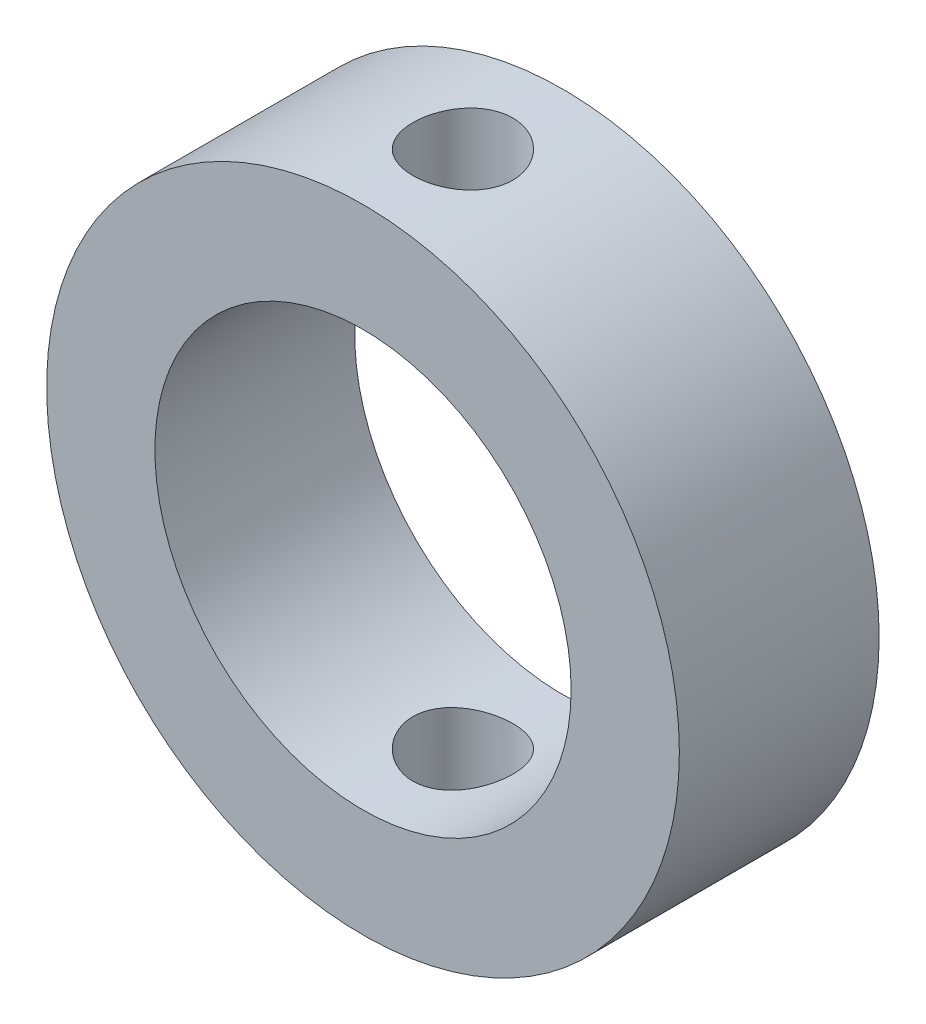
ISO-10303-21;
HEADER;
FILE_DESCRIPTION(('STEP AP214'),'2;1');
FILE_NAME('part.step','',(''),(''),'','','');
FILE_SCHEMA(('AUTOMOTIVE_DESIGN { 1 0 10303 214 1 1 1 1 }'));
ENDSEC;
DATA;
#1=APPLICATION_CONTEXT('core data for automotive mechanical design processes');
#2=APPLICATION_PROTOCOL_DEFINITION('international standard','automotive_design',2000,#1);
#3=PRODUCT_CONTEXT('',#1,'mechanical');
#4=PRODUCT('Part','Part','',(#3));
#5=PRODUCT_RELATED_PRODUCT_CATEGORY('part','',(#4));
#6=PRODUCT_DEFINITION_FORMATION('','',#4);
#7=PRODUCT_DEFINITION_CONTEXT('part definition',#1,'design');
#8=PRODUCT_DEFINITION('design','',#6,#7);
#9=PRODUCT_DEFINITION_SHAPE('','',#8);
#10=(LENGTH_UNIT() NAMED_UNIT(*) SI_UNIT(.MILLI.,.METRE.));
#11=(NAMED_UNIT(*) PLANE_ANGLE_UNIT() SI_UNIT($,.RADIAN.));
#12=(NAMED_UNIT(*) SI_UNIT($,.STERADIAN.) SOLID_ANGLE_UNIT());
#13=UNCERTAINTY_MEASURE_WITH_UNIT(LENGTH_MEASURE(1.E-05),#10,'distance_accuracy_value','');
#14=(GEOMETRIC_REPRESENTATION_CONTEXT(3) GLOBAL_UNCERTAINTY_ASSIGNED_CONTEXT((#13)) GLOBAL_UNIT_ASSIGNED_CONTEXT((#10,
#11,#12)) REPRESENTATION_CONTEXT('',''));
#15=CARTESIAN_POINT('',(0.,0.,0.));
#16=DIRECTION('',(0.,0.,1.));
#17=DIRECTION('',(1.,0.,0.));
#18=AXIS2_PLACEMENT_3D('',#15,#16,#17);
#19=CARTESIAN_POINT('',(0.,0.,12.));
#20=DIRECTION('',(0.,0.,1.));
#21=DIRECTION('',(1.,0.,0.));
#22=AXIS2_PLACEMENT_3D('',#19,#20,#21);
#23=PLANE('',#22);
#24=CARTESIAN_POINT('',(0.,0.,12.));
#25=DIRECTION('',(0.,0.,1.));
#26=DIRECTION('',(1.,0.,0.));
#27=AXIS2_PLACEMENT_3D('',#24,#25,#26);
#28=CIRCLE('',#27,19.);
#29=CARTESIAN_POINT('',(19.,0.,12.));
#30=VERTEX_POINT('',#29);
#31=EDGE_CURVE('E10',#30,#30,#28,.T.);
#32=ORIENTED_EDGE('',*,*,#31,.T.);
#33=EDGE_LOOP('',(#32));
#34=FACE_BOUND('',#33,.T.);
#35=CARTESIAN_POINT('',(0.,0.,12.));
#36=DIRECTION('',(0.,0.,1.));
#37=DIRECTION('',(1.,0.,0.));
#38=AXIS2_PLACEMENT_3D('',#35,#36,#37);
#39=CIRCLE('',#38,12.5);
#40=CARTESIAN_POINT('',(12.5,0.,12.));
#41=VERTEX_POINT('',#40);
#42=EDGE_CURVE('E57',#41,#41,#39,.T.);
#43=ORIENTED_EDGE('',*,*,#42,.F.);
#44=EDGE_LOOP('',(#43));
#45=FACE_BOUND('',#44,.T.);
#46=ADVANCED_FACE('F40',(#34,#45),#23,.T.);
#47=CARTESIAN_POINT('',(0.,0.,0.));
#48=DIRECTION('',(0.,0.,1.));
#49=DIRECTION('',(1.,0.,0.));
#50=AXIS2_PLACEMENT_3D('',#47,#48,#49);
#51=PLANE('',#50);
#52=CARTESIAN_POINT('',(0.,0.,0.));
#53=DIRECTION('',(0.,0.,1.));
#54=DIRECTION('',(1.,0.,0.));
#55=AXIS2_PLACEMENT_3D('',#52,#53,#54);
#56=CIRCLE('',#55,19.);
#57=CARTESIAN_POINT('',(19.,0.,0.));
#58=VERTEX_POINT('',#57);
#59=EDGE_CURVE('E51',#58,#58,#56,.T.);
#60=ORIENTED_EDGE('',*,*,#59,.F.);
#61=EDGE_LOOP('',(#60));
#62=FACE_BOUND('',#61,.T.);
#63=CARTESIAN_POINT('',(0.,0.,0.));
#64=DIRECTION('',(0.,0.,1.));
#65=DIRECTION('',(1.,0.,0.));
#66=AXIS2_PLACEMENT_3D('',#63,#64,#65);
#67=CIRCLE('',#66,12.5);
#68=CARTESIAN_POINT('',(12.5,0.,0.));
#69=VERTEX_POINT('',#68);
#70=EDGE_CURVE('E56',#69,#69,#67,.T.);
#71=ORIENTED_EDGE('',*,*,#70,.T.);
#72=EDGE_LOOP('',(#71));
#73=FACE_BOUND('',#72,.T.);
#74=ADVANCED_FACE('F92',(#62,#73),#51,.F.);
#75=CARTESIAN_POINT('',(0.,0.,12.));
#76=DIRECTION('',(0.,0.,-1.));
#77=DIRECTION('',(-1.,0.,0.));
#78=AXIS2_PLACEMENT_3D('',#75,#76,#77);
#79=CYLINDRICAL_SURFACE('',#78,19.);
#80=CARTESIAN_POINT('',(0.,-19.,9.));
#81=CARTESIAN_POINT('',(0.167395200213044,-18.9999972240724,8.99999318150179));
#82=CARTESIAN_POINT('',(0.334884874788033,-18.9977646846382,8.98594210979435));
#83=CARTESIAN_POINT('',(0.665175270422548,-18.9890735602357,8.93012751306062));
#84=CARTESIAN_POINT('',(0.827971389790523,-18.9826109658894,8.88833769585688));
#85=CARTESIAN_POINT('',(1.14404753345886,-18.9661853440085,8.77833164300608));
#86=CARTESIAN_POINT('',(1.2973349148092,-18.9562250634571,8.71013614133113));
#87=CARTESIAN_POINT('',(1.59026942093823,-18.9339021624185,8.54930690892295));
#88=CARTESIAN_POINT('',(1.72991828221782,-18.9215398483668,8.45667629492092));
#89=CARTESIAN_POINT('',(1.99283693302404,-18.895666487681,8.24875622900043));
#90=CARTESIAN_POINT('',(2.11597212000229,-18.8821473182235,8.13329756247262));
#91=CARTESIAN_POINT('',(2.34120609409226,-18.8555468666848,7.88336303658814));
#92=CARTESIAN_POINT('',(2.44330361812925,-18.8424656109348,7.74888603621164));
#93=CARTESIAN_POINT('',(2.6240952801003,-18.8181433723965,7.46381831106108));
#94=CARTESIAN_POINT('',(2.70265784849318,-18.8069128876018,7.31314317048161));
#95=CARTESIAN_POINT('',(2.83330843623881,-18.7876755172578,7.00052865042408));
#96=CARTESIAN_POINT('',(2.88539805669314,-18.779668436761,6.83858995284711));
#97=CARTESIAN_POINT('',(2.9612032507172,-18.767864811149,6.50946610209667));
#98=CARTESIAN_POINT('',(2.98515018535338,-18.764033952474,6.34233549043282));
#99=CARTESIAN_POINT('',(3.00470725611049,-18.7609125219047,6.00638765388364));
#100=CARTESIAN_POINT('',(3.00031919304727,-18.7616216614731,5.83757053686414));
#101=CARTESIAN_POINT('',(2.96351961421685,-18.76746874767,5.50468405688764));
#102=CARTESIAN_POINT('',(2.93136679776229,-18.7725658083082,5.34058527341682));
#103=CARTESIAN_POINT('',(2.8403558507158,-18.7865504980478,5.02014120785184));
#104=CARTESIAN_POINT('',(2.78149689033187,-18.79543824493,4.86379616684323));
#105=CARTESIAN_POINT('',(2.6384785155272,-18.8160475867562,4.56251637450162));
#106=CARTESIAN_POINT('',(2.55421051731569,-18.8277813007915,4.4176340312379));
#107=CARTESIAN_POINT('',(2.3628433457816,-18.852751887079,4.14396789581904));
#108=CARTESIAN_POINT('',(2.25574251495398,-18.8659888684252,4.01518527346906));
#109=CARTESIAN_POINT('',(2.02033468405641,-18.8926547085158,3.77587576680137));
#110=CARTESIAN_POINT('',(1.89180547305152,-18.9060840660713,3.66556740906069));
#111=CARTESIAN_POINT('',(1.61794401566889,-18.9314853396994,3.46805215714333));
#112=CARTESIAN_POINT('',(1.47261168060432,-18.943457248079,3.38084538490472));
#113=CARTESIAN_POINT('',(1.16907261376921,-18.9646092293985,3.23199357249975));
#114=CARTESIAN_POINT('',(1.01085691624053,-18.9737873366695,3.17036651873699));
#115=CARTESIAN_POINT('',(0.686144192781849,-18.9883014789364,3.07461938599573));
#116=CARTESIAN_POINT('',(0.519647788837096,-18.9936378020341,3.04049724435513));
#117=CARTESIAN_POINT('',(0.184984736062192,-18.9998286919511,3.0010217261686));
#118=CARTESIAN_POINT('',(0.0168543348027385,-19.0007300274,2.9953681231511));
#119=CARTESIAN_POINT('',(-0.317952531425077,-18.9980770575087,3.01219164968731));
#120=CARTESIAN_POINT('',(-0.484629046224454,-18.9945229054864,3.03466781126644));
#121=CARTESIAN_POINT('',(-0.810879134741272,-18.9833872413873,3.10686316263139));
#122=CARTESIAN_POINT('',(-0.970486125590159,-18.9758275205639,3.15643499115847));
#123=CARTESIAN_POINT('',(-1.27912372239425,-18.9575252911701,3.28125833514596));
#124=CARTESIAN_POINT('',(-1.42815378551392,-18.9467826193886,3.35651116747288));
#125=CARTESIAN_POINT('',(-1.71271987736475,-18.9231911639978,3.531256990221));
#126=CARTESIAN_POINT('',(-1.84813841462226,-18.9103262188696,3.6309390875747));
#127=CARTESIAN_POINT('',(-2.10043218264525,-18.883969518103,3.85145200517811));
#128=CARTESIAN_POINT('',(-2.21730621147132,-18.8704777219092,3.97228419517836));
#129=CARTESIAN_POINT('',(-2.43029521840863,-18.8442382720014,4.23300853112575));
#130=CARTESIAN_POINT('',(-2.52620819677151,-18.8314986550647,4.37306662717604));
#131=CARTESIAN_POINT('',(-2.69314533298653,-18.8083518860728,4.66748262453215));
#132=CARTESIAN_POINT('',(-2.76417021883834,-18.7979446657959,4.82184010740069));
#133=CARTESIAN_POINT('',(-2.87900699225531,-18.7807002117535,5.13988822187714));
#134=CARTESIAN_POINT('',(-2.92292252251651,-18.7738493975614,5.30354066232477));
#135=CARTESIAN_POINT('',(-2.98262220399549,-18.7644582567649,5.6360153344807));
#136=CARTESIAN_POINT('',(-2.99840852776725,-18.7619175972673,5.80483716590752));
#137=CARTESIAN_POINT('',(-3.0013458746632,-18.7614477526913,6.14084334598222));
#138=CARTESIAN_POINT('',(-2.98881465767375,-18.7634673948558,6.30802493116096));
#139=CARTESIAN_POINT('',(-2.93615642039242,-18.7717789448073,6.63787026604105));
#140=CARTESIAN_POINT('',(-2.89602946421833,-18.778070842668,6.80053402623851));
#141=CARTESIAN_POINT('',(-2.78943553807322,-18.794199354287,7.11662212969122));
#142=CARTESIAN_POINT('',(-2.72299316138579,-18.804032657621,7.27005494601528));
#143=CARTESIAN_POINT('',(-2.56568649491816,-18.8261396450455,7.56364713665079));
#144=CARTESIAN_POINT('',(-2.47482119948363,-18.8384134296215,7.70380596406221));
#145=CARTESIAN_POINT('',(-2.27010290160429,-18.8641819165768,7.96848193612583));
#146=CARTESIAN_POINT('',(-2.15601525457361,-18.8776882356084,8.09281648317715));
#147=CARTESIAN_POINT('',(-1.90858649068852,-18.9043049971159,8.32068696110511));
#148=CARTESIAN_POINT('',(-1.77524092123377,-18.9174153471904,8.42421806876997));
#149=CARTESIAN_POINT('',(-1.49211329897017,-18.9418556038111,8.608117130421));
#150=CARTESIAN_POINT('',(-1.34223536218177,-18.9531740853537,8.68833897434538));
#151=CARTESIAN_POINT('',(-1.03101937641098,-18.9726437984251,8.82234719309167));
#152=CARTESIAN_POINT('',(-0.869693179799288,-18.9807982506767,8.87616046453452));
#153=CARTESIAN_POINT('',(-0.589739099355735,-18.9911973335544,8.9438581821044));
#154=CARTESIAN_POINT('',(-0.472823930142805,-18.9944810635349,8.96487848383233));
#155=CARTESIAN_POINT('',(-0.237288316828361,-18.9988833649697,8.99295170816852));
#156=CARTESIAN_POINT('',(-0.118667897525957,-19.000001967879,9.00000483369205));
#157=CARTESIAN_POINT('',(0.,-19.,9.));
#158=B_SPLINE_CURVE_WITH_KNOTS('',3,(#80,#81,#82,#83,#84,#85,#86,#87,#88,#89,#90,#91,#92,#93,
#94,#95,#96,#97,#98,#99,#100,#101,#102,#103,#104,#105,#106,#107,#108,#109,#110,#111,#112,#113,
#114,#115,#116,#117,#118,#119,#120,#121,#122,#123,#124,#125,#126,#127,#128,#129,#130,#131,#132,
#133,#134,#135,#136,#137,#138,#139,#140,#141,#142,#143,#144,#145,#146,#147,#148,#149,#150,#151,
#152,#153,#154,#155,#156,#157),.UNSPECIFIED.,.T.,.F.,(4,2,2,2,2,2,2,2,2,2,2,2,2,2,2,2,2,2,2,2,2,
2,2,2,2,2,2,2,2,2,2,2,2,2,2,2,2,2,4),(0.,0.501751911412535,1.00398008893817,1.50581470964933,
2.00758535160925,2.51322514893025,3.01889529538689,3.52734173016572,4.0357574101042,
4.5399634980397,5.04413754173826,5.54366399670822,6.04320597362876,6.54491371515846,
7.04665788959371,7.55397191335254,8.06128861483534,8.56896143470457,9.07659617937734,
9.57886607695304,10.0811186913724,10.5806665697856,11.0802400677869,11.583810193871,
12.0874129449106,12.5956735489114,13.1039192845792,13.6102096956392,14.1164610017594,
14.6170597501047,15.1176573353292,15.6177881828935,16.1179396273336,16.6234208130271,
17.1290190580601,17.6377213704247,18.1459044984556,18.5016059126814,18.8573021592355),.UNSPECIFIED.);
#159=CARTESIAN_POINT('',(0.,-19.,9.));
#160=VERTEX_POINT('',#159);
#161=EDGE_CURVE('E82',#160,#160,#158,.T.);
#162=ORIENTED_EDGE('',*,*,#161,.T.);
#163=EDGE_LOOP('',(#162));
#164=FACE_BOUND('',#163,.T.);
#165=CARTESIAN_POINT('',(0.,19.,9.));
#166=CARTESIAN_POINT('',(-0.167395200213042,18.9999972240724,8.99999318150179));
#167=CARTESIAN_POINT('',(-0.334884874788031,18.9977646846382,8.98594210979435));
#168=CARTESIAN_POINT('',(-0.665175270422546,18.9890735602357,8.93012751306062));
#169=CARTESIAN_POINT('',(-0.827971389790521,18.9826109658894,8.88833769585688));
#170=CARTESIAN_POINT('',(-1.14404753345886,18.9661853440085,8.77833164300608));
#171=CARTESIAN_POINT('',(-1.2973349148092,18.9562250634571,8.71013614133113));
#172=CARTESIAN_POINT('',(-1.59026942093823,18.9339021624185,8.54930690892295));
#173=CARTESIAN_POINT('',(-1.72991828221782,18.9215398483668,8.45667629492092));
#174=CARTESIAN_POINT('',(-1.99283693302403,18.895666487681,8.24875622900043));
#175=CARTESIAN_POINT('',(-2.11597212000228,18.8821473182235,8.13329756247262));
#176=CARTESIAN_POINT('',(-2.34120609409226,18.8555468666848,7.88336303658814));
#177=CARTESIAN_POINT('',(-2.44330361812924,18.8424656109348,7.74888603621163));
#178=CARTESIAN_POINT('',(-2.6240952801003,18.8181433723965,7.46381831106108));
#179=CARTESIAN_POINT('',(-2.70265784849317,18.8069128876018,7.31314317048161));
#180=CARTESIAN_POINT('',(-2.83330843623881,18.7876755172578,7.00052865042408));
#181=CARTESIAN_POINT('',(-2.88539805669313,18.779668436761,6.83858995284711));
#182=CARTESIAN_POINT('',(-2.96120325071719,18.767864811149,6.50946610209667));
#183=CARTESIAN_POINT('',(-2.98515018535337,18.764033952474,6.34233549043282));
#184=CARTESIAN_POINT('',(-3.00470725611048,18.7609125219047,6.00638765388364));
#185=CARTESIAN_POINT('',(-3.00031919304727,18.7616216614731,5.83757053686414));
#186=CARTESIAN_POINT('',(-2.96351961421685,18.76746874767,5.50468405688764));
#187=CARTESIAN_POINT('',(-2.93136679776228,18.7725658083082,5.34058527341682));
#188=CARTESIAN_POINT('',(-2.84035585071579,18.7865504980478,5.02014120785184));
#189=CARTESIAN_POINT('',(-2.78149689033187,18.79543824493,4.86379616684323));
#190=CARTESIAN_POINT('',(-2.63847851552719,18.8160475867562,4.56251637450161));
#191=CARTESIAN_POINT('',(-2.55421051731569,18.8277813007915,4.41763403123789));
#192=CARTESIAN_POINT('',(-2.36284334578159,18.852751887079,4.14396789581904));
#193=CARTESIAN_POINT('',(-2.25574251495398,18.8659888684252,4.01518527346906));
#194=CARTESIAN_POINT('',(-2.02033468405641,18.8926547085158,3.77587576680136));
#195=CARTESIAN_POINT('',(-1.89180547305151,18.9060840660713,3.66556740906069));
#196=CARTESIAN_POINT('',(-1.61794401566888,18.9314853396994,3.46805215714332));
#197=CARTESIAN_POINT('',(-1.47261168060432,18.943457248079,3.38084538490472));
#198=CARTESIAN_POINT('',(-1.1690726137692,18.9646092293985,3.23199357249975));
#199=CARTESIAN_POINT('',(-1.01085691624053,18.9737873366695,3.17036651873699));
#200=CARTESIAN_POINT('',(-0.686144192781842,18.9883014789364,3.07461938599573));
#201=CARTESIAN_POINT('',(-0.51964778883709,18.9936378020341,3.04049724435513));
#202=CARTESIAN_POINT('',(-0.184984736062187,18.9998286919511,3.0010217261686));
#203=CARTESIAN_POINT('',(-0.0168543348027339,19.0007300274,2.9953681231511));
#204=CARTESIAN_POINT('',(0.317952531425082,18.9980770575087,3.01219164968731));
#205=CARTESIAN_POINT('',(0.484629046224459,18.9945229054864,3.03466781126644));
#206=CARTESIAN_POINT('',(0.810879134741278,18.9833872413873,3.10686316263139));
#207=CARTESIAN_POINT('',(0.970486125590166,18.9758275205639,3.15643499115847));
#208=CARTESIAN_POINT('',(1.27912372239425,18.9575252911701,3.28125833514596));
#209=CARTESIAN_POINT('',(1.42815378551393,18.9467826193886,3.35651116747288));
#210=CARTESIAN_POINT('',(1.71271987736476,18.9231911639978,3.531256990221));
#211=CARTESIAN_POINT('',(1.84813841462226,18.9103262188696,3.6309390875747));
#212=CARTESIAN_POINT('',(2.10043218264526,18.883969518103,3.85145200517811));
#213=CARTESIAN_POINT('',(2.21730621147133,18.8704777219092,3.97228419517836));
#214=CARTESIAN_POINT('',(2.43029521840863,18.8442382720014,4.23300853112576));
#215=CARTESIAN_POINT('',(2.52620819677152,18.8314986550647,4.37306662717604));
#216=CARTESIAN_POINT('',(2.69314533298653,18.8083518860728,4.66748262453215));
#217=CARTESIAN_POINT('',(2.76417021883834,18.7979446657959,4.82184010740069));
#218=CARTESIAN_POINT('',(2.87900699225531,18.7807002117535,5.13988822187714));
#219=CARTESIAN_POINT('',(2.92292252251651,18.7738493975614,5.30354066232477));
#220=CARTESIAN_POINT('',(2.9826222039955,18.7644582567649,5.6360153344807));
#221=CARTESIAN_POINT('',(2.99840852776725,18.7619175972673,5.80483716590753));
#222=CARTESIAN_POINT('',(3.0013458746632,18.7614477526913,6.14084334598222));
#223=CARTESIAN_POINT('',(2.98881465767375,18.7634673948558,6.30802493116096));
#224=CARTESIAN_POINT('',(2.93615642039242,18.7717789448073,6.63787026604105));
#225=CARTESIAN_POINT('',(2.89602946421833,18.778070842668,6.80053402623851));
#226=CARTESIAN_POINT('',(2.78943553807322,18.794199354287,7.11662212969122));
#227=CARTESIAN_POINT('',(2.72299316138579,18.804032657621,7.27005494601528));
#228=CARTESIAN_POINT('',(2.56568649491816,18.8261396450455,7.5636471366508));
#229=CARTESIAN_POINT('',(2.47482119948363,18.8384134296215,7.70380596406221));
#230=CARTESIAN_POINT('',(2.27010290160429,18.8641819165768,7.96848193612583));
#231=CARTESIAN_POINT('',(2.15601525457361,18.8776882356084,8.09281648317715));
#232=CARTESIAN_POINT('',(1.90858649068852,18.9043049971159,8.32068696110511));
#233=CARTESIAN_POINT('',(1.77524092123377,18.9174153471904,8.42421806876997));
#234=CARTESIAN_POINT('',(1.49211329897017,18.9418556038111,8.60811713042101));
#235=CARTESIAN_POINT('',(1.34223536218178,18.9531740853537,8.68833897434538));
#236=CARTESIAN_POINT('',(1.03101937641098,18.9726437984251,8.82234719309167));
#237=CARTESIAN_POINT('',(0.869693179799289,18.9807982506767,8.87616046453453));
#238=CARTESIAN_POINT('',(0.589739099355737,18.9911973335544,8.9438581821044));
#239=CARTESIAN_POINT('',(0.472823930142806,18.9944810635349,8.96487848383233));
#240=CARTESIAN_POINT('',(0.237288316828362,18.9988833649697,8.99295170816852));
#241=CARTESIAN_POINT('',(0.118667897525959,19.000001967879,9.00000483369205));
#242=CARTESIAN_POINT('',(0.,19.,9.));
#243=B_SPLINE_CURVE_WITH_KNOTS('',3,(#165,#166,#167,#168,#169,#170,#171,#172,#173,#174,#175,
#176,#177,#178,#179,#180,#181,#182,#183,#184,#185,#186,#187,#188,#189,#190,#191,#192,#193,#194,
#195,#196,#197,#198,#199,#200,#201,#202,#203,#204,#205,#206,#207,#208,#209,#210,#211,#212,#213,
#214,#215,#216,#217,#218,#219,#220,#221,#222,#223,#224,#225,#226,#227,#228,#229,#230,#231,#232,
#233,#234,#235,#236,#237,#238,#239,#240,#241,#242),.UNSPECIFIED.,.T.,.F.,(4,2,2,2,2,2,2,2,2,2,2,
2,2,2,2,2,2,2,2,2,2,2,2,2,2,2,2,2,2,2,2,2,2,2,2,2,2,2,4),(0.,0.501751911412535,1.00398008893817,
1.50581470964933,2.00758535160925,2.51322514893025,3.01889529538689,3.52734173016572,
4.0357574101042,4.5399634980397,5.04413754173826,5.54366399670822,6.04320597362876,
6.54491371515846,7.04665788959372,7.55397191335254,8.06128861483534,8.56896143470457,
9.07659617937734,9.57886607695304,10.0811186913724,10.5806665697856,11.0802400677869,
11.583810193871,12.0874129449107,12.5956735489114,13.1039192845792,13.6102096956392,
14.1164610017594,14.6170597501047,15.1176573353293,15.6177881828935,16.1179396273336,
16.6234208130271,17.1290190580601,17.6377213704247,18.1459044984556,18.5016059126814,
18.8573021592355),.UNSPECIFIED.);
#244=CARTESIAN_POINT('',(0.,19.,9.));
#245=VERTEX_POINT('',#244);
#246=EDGE_CURVE('E76',#245,#245,#243,.T.);
#247=ORIENTED_EDGE('',*,*,#246,.T.);
#248=EDGE_LOOP('',(#247));
#249=FACE_BOUND('',#248,.T.);
#250=ORIENTED_EDGE('',*,*,#31,.F.);
#251=EDGE_LOOP('',(#250));
#252=FACE_BOUND('',#251,.T.);
#253=ORIENTED_EDGE('',*,*,#59,.T.);
#254=EDGE_LOOP('',(#253));
#255=FACE_BOUND('',#254,.T.);
#256=ADVANCED_FACE('F39',(#164,#249,#252,#255),#79,.T.);
#257=CARTESIAN_POINT('',(0.,0.,12.));
#258=DIRECTION('',(0.,0.,-1.));
#259=DIRECTION('',(-1.,0.,0.));
#260=AXIS2_PLACEMENT_3D('',#257,#258,#259);
#261=CYLINDRICAL_SURFACE('',#260,12.5);
#262=CARTESIAN_POINT('',(0.,-12.5,9.));
#263=CARTESIAN_POINT('',(0.165963929028718,-12.4999970714968,8.99999497592274));
#264=CARTESIAN_POINT('',(0.331985420928069,-12.4966615634859,8.98618158976393));
#265=CARTESIAN_POINT('',(0.659284290971381,-12.4836783946933,8.93136726040462));
#266=CARTESIAN_POINT('',(0.820558683214276,-12.4740268462166,8.89034957200532));
#267=CARTESIAN_POINT('',(1.13358839471402,-12.4494823208195,8.78250766549565));
#268=CARTESIAN_POINT('',(1.28535442324823,-12.4345953702841,8.71571311014241));
#269=CARTESIAN_POINT('',(1.57552517879763,-12.4011725442513,8.55831456355411));
#270=CARTESIAN_POINT('',(1.71392971475166,-12.3826366165873,8.46771023192273));
#271=CARTESIAN_POINT('',(1.97609263393972,-12.3435386014785,8.26343582162447));
#272=CARTESIAN_POINT('',(2.0995595210048,-12.3229472454311,8.14939721895074));
#273=CARTESIAN_POINT('',(2.32581080811943,-12.2822574370147,7.90228113093536));
#274=CARTESIAN_POINT('',(2.42859304624489,-12.2621590363612,7.76920165795905));
#275=CARTESIAN_POINT('',(2.61189993555015,-12.224437969062,7.48555416698254));
#276=CARTESIAN_POINT('',(2.69210377047565,-12.2068525815312,7.33477341624116));
#277=CARTESIAN_POINT('',(2.82591582947333,-12.1765733412448,7.02138016487152));
#278=CARTESIAN_POINT('',(2.87952794169564,-12.1638787734309,6.85876939797685));
#279=CARTESIAN_POINT('',(2.95765058108663,-12.1451184675007,6.5295234267311));
#280=CARTESIAN_POINT('',(2.98268262400617,-12.1389341034343,6.36301887847449));
#281=CARTESIAN_POINT('',(3.00455808879087,-12.1335389605945,6.02806762035724));
#282=CARTESIAN_POINT('',(3.00140571682399,-12.1343271412568,5.85962120404308));
#283=CARTESIAN_POINT('',(2.96741912081942,-12.1426811387008,5.52952403398712));
#284=CARTESIAN_POINT('',(2.93720103400494,-12.1500960921292,5.36780543481044));
#285=CARTESIAN_POINT('',(2.85092141637189,-12.1706283738785,5.05180268335217));
#286=CARTESIAN_POINT('',(2.79485817372027,-12.1837460799133,4.89751902426557));
#287=CARTESIAN_POINT('',(2.65794121231782,-12.2143476734445,4.59908702191564));
#288=CARTESIAN_POINT('',(2.5768594824696,-12.2318714325758,4.45504754708331));
#289=CARTESIAN_POINT('',(2.39236688956383,-12.2692875046197,4.18239549927742));
#290=CARTESIAN_POINT('',(2.28895240342647,-12.2891802016137,4.05378543471489));
#291=CARTESIAN_POINT('',(2.05951493908847,-12.329732025739,3.81210642968126));
#292=CARTESIAN_POINT('',(1.93297064389908,-12.3503975788014,3.69953290093779));
#293=CARTESIAN_POINT('',(1.66255592459692,-12.3896951594929,3.49711528025362));
#294=CARTESIAN_POINT('',(1.51868504982141,-12.4083271342049,3.40727177970739));
#295=CARTESIAN_POINT('',(1.21702847718581,-12.4415394956922,3.25270277938722));
#296=CARTESIAN_POINT('',(1.05920278696054,-12.4561077058019,3.18805254376221));
#297=CARTESIAN_POINT('',(0.734497606078677,-12.4794620474154,3.08633492095141));
#298=CARTESIAN_POINT('',(0.567619713387663,-12.4882491958651,3.04926268237319));
#299=CARTESIAN_POINT('',(0.233787399651666,-12.4989027542709,3.00449793534796));
#300=CARTESIAN_POINT('',(0.0669284805450091,-12.5009282130753,2.99613010753843));
#301=CARTESIAN_POINT('',(-0.265804381586628,-12.4982807419474,3.0071667668509));
#302=CARTESIAN_POINT('',(-0.431678404764951,-12.4936083648176,3.02656896198723));
#303=CARTESIAN_POINT('',(-0.755422580108845,-12.4781916395217,3.09203697851638));
#304=CARTESIAN_POINT('',(-0.913370579311302,-12.4675301590363,3.1377391095738));
#305=CARTESIAN_POINT('',(-1.21935330013476,-12.4413335015664,3.25409819169527));
#306=CARTESIAN_POINT('',(-1.3673870666415,-12.4257978558334,3.32475754297811));
#307=CARTESIAN_POINT('',(-1.6520615099557,-12.3911910149582,3.49036659359785));
#308=CARTESIAN_POINT('',(-1.78847176740355,-12.3720653178033,3.58570071692437));
#309=CARTESIAN_POINT('',(-2.04359904096632,-12.3324936406987,3.79745692901341));
#310=CARTESIAN_POINT('',(-2.16231325074336,-12.3120474520734,3.91388235608078));
#311=CARTESIAN_POINT('',(-2.38142453789941,-12.2715742142771,4.16764083120855));
#312=CARTESIAN_POINT('',(-2.48134974047369,-12.2515669262668,4.3053851220821));
#313=CARTESIAN_POINT('',(-2.65666020824081,-12.2147538797452,4.59609042789673));
#314=CARTESIAN_POINT('',(-2.7320465722335,-12.1979479778962,4.74905076109347));
#315=CARTESIAN_POINT('',(-2.85558993518171,-12.1696189519335,5.06501251354399));
#316=CARTESIAN_POINT('',(-2.90390754385905,-12.1580647463107,5.22794820342123));
#317=CARTESIAN_POINT('',(-2.97238380283978,-12.1415072663683,5.55994618502069));
#318=CARTESIAN_POINT('',(-2.99254804274991,-12.1365026916888,5.72900725376178));
#319=CARTESIAN_POINT('',(-3.00387066449353,-12.1337046220624,6.0636707002806));
#320=CARTESIAN_POINT('',(-2.99578106592266,-12.1357241633848,6.2292464963267));
#321=CARTESIAN_POINT('',(-2.95253345626267,-12.1463176460425,6.55659976422369));
#322=CARTESIAN_POINT('',(-2.91737590900096,-12.1548914750658,6.71837730111136));
#323=CARTESIAN_POINT('',(-2.82138591303537,-12.1775274976748,7.03279755254825));
#324=CARTESIAN_POINT('',(-2.76068402045612,-12.191561756094,7.18548227258375));
#325=CARTESIAN_POINT('',(-2.61543373580582,-12.2235433612686,7.47860441388369));
#326=CARTESIAN_POINT('',(-2.53088229934855,-12.2414912075257,7.61904026858635));
#327=CARTESIAN_POINT('',(-2.33793007708463,-12.279819325529,7.88733700011951));
#328=CARTESIAN_POINT('',(-2.22900267979018,-12.3002478697533,8.01481232309873));
#329=CARTESIAN_POINT('',(-1.99143074773236,-12.3409359831145,8.24991998805192));
#330=CARTESIAN_POINT('',(-1.86278158874234,-12.361195511444,8.35754766321024));
#331=CARTESIAN_POINT('',(-1.5868829988014,-12.3996570299581,8.55160925955474));
#332=CARTESIAN_POINT('',(-1.43936414359402,-12.4178200201219,8.637668405442));
#333=CARTESIAN_POINT('',(-1.13153622828567,-12.4496380610582,8.78362953274789));
#334=CARTESIAN_POINT('',(-0.971236973691219,-12.4632965272855,8.84355134339162));
#335=CARTESIAN_POINT('',(-0.675887025694765,-12.4824059901497,8.92603862513779));
#336=CARTESIAN_POINT('',(-0.542312066268422,-12.4889599449579,8.9537166157857));
#337=CARTESIAN_POINT('',(-0.272504227478249,-12.4977580149525,8.99069878085188));
#338=CARTESIAN_POINT('',(-0.136271517915776,-12.5000024045682,9.00000412522552));
#339=CARTESIAN_POINT('',(0.,-12.5,9.));
#340=B_SPLINE_CURVE_WITH_KNOTS('',3,(#262,#263,#264,#265,#266,#267,#268,#269,#270,#271,#272,
#273,#274,#275,#276,#277,#278,#279,#280,#281,#282,#283,#284,#285,#286,#287,#288,#289,#290,#291,
#292,#293,#294,#295,#296,#297,#298,#299,#300,#301,#302,#303,#304,#305,#306,#307,#308,#309,#310,
#311,#312,#313,#314,#315,#316,#317,#318,#319,#320,#321,#322,#323,#324,#325,#326,#327,#328,#329,
#330,#331,#332,#333,#334,#335,#336,#337,#338,#339),.UNSPECIFIED.,.T.,.F.,(4,2,2,2,2,2,2,2,2,2,2,
2,2,2,2,2,2,2,2,2,2,2,2,2,2,2,2,2,2,2,2,2,2,2,2,2,2,2,4),(0.,0.497392599366678,
0.995091645758824,1.49221966408501,1.98935478998519,2.49500570148357,3.00070943533306,
3.51327262050848,4.02576083835037,4.52873995359111,5.03164400680465,5.52338274964838,
6.01515406709138,6.51154667521171,7.00801987450003,7.51749958381935,8.0269925475217,
8.53799614678203,9.04890983140415,9.54771776810825,10.0464845383097,10.5385143736981,
11.0305915421211,11.5308523313794,12.031192370573,12.5427824523192,13.0543496229377,
13.5628484119093,14.0712462285018,14.5662165454702,15.0611783809799,15.5536406351284,
16.0461657803879,16.5505844610431,17.0551215958269,17.5678974206352,18.0802835459069,
18.4887142303991,18.897118905514),.UNSPECIFIED.);
#341=CARTESIAN_POINT('',(0.,-12.5,9.));
#342=VERTEX_POINT('',#341);
#343=EDGE_CURVE('E45',#342,#342,#340,.T.);
#344=ORIENTED_EDGE('',*,*,#343,.F.);
#345=EDGE_LOOP('',(#344));
#346=FACE_BOUND('',#345,.T.);
#347=CARTESIAN_POINT('',(0.,12.5,9.));
#348=CARTESIAN_POINT('',(-0.165963929028714,12.4999970714968,8.99999497592274));
#349=CARTESIAN_POINT('',(-0.331985420928066,12.4966615634859,8.98618158976393));
#350=CARTESIAN_POINT('',(-0.659284290971378,12.4836783946933,8.93136726040462));
#351=CARTESIAN_POINT('',(-0.820558683214273,12.4740268462166,8.89034957200532));
#352=CARTESIAN_POINT('',(-1.13358839471401,12.4494823208195,8.78250766549565));
#353=CARTESIAN_POINT('',(-1.28535442324822,12.4345953702841,8.71571311014241));
#354=CARTESIAN_POINT('',(-1.57552517879763,12.4011725442513,8.55831456355411));
#355=CARTESIAN_POINT('',(-1.71392971475166,12.3826366165873,8.46771023192274));
#356=CARTESIAN_POINT('',(-1.97609263393972,12.3435386014785,8.26343582162447));
#357=CARTESIAN_POINT('',(-2.0995595210048,12.3229472454311,8.14939721895074));
#358=CARTESIAN_POINT('',(-2.32581080811943,12.2822574370147,7.90228113093536));
#359=CARTESIAN_POINT('',(-2.42859304624489,12.2621590363612,7.76920165795905));
#360=CARTESIAN_POINT('',(-2.61189993555015,12.224437969062,7.48555416698254));
#361=CARTESIAN_POINT('',(-2.69210377047565,12.2068525815312,7.33477341624116));
#362=CARTESIAN_POINT('',(-2.82591582947332,12.1765733412448,7.02138016487152));
#363=CARTESIAN_POINT('',(-2.87952794169564,12.1638787734309,6.85876939797685));
#364=CARTESIAN_POINT('',(-2.95765058108663,12.1451184675007,6.5295234267311));
#365=CARTESIAN_POINT('',(-2.98268262400616,12.1389341034343,6.36301887847449));
#366=CARTESIAN_POINT('',(-3.00455808879087,12.1335389605945,6.02806762035724));
#367=CARTESIAN_POINT('',(-3.00140571682399,12.1343271412568,5.85962120404308));
#368=CARTESIAN_POINT('',(-2.96741912081942,12.1426811387008,5.52952403398712));
#369=CARTESIAN_POINT('',(-2.93720103400494,12.1500960921292,5.36780543481045));
#370=CARTESIAN_POINT('',(-2.85092141637188,12.1706283738785,5.05180268335217));
#371=CARTESIAN_POINT('',(-2.79485817372027,12.1837460799133,4.89751902426557));
#372=CARTESIAN_POINT('',(-2.65794121231782,12.2143476734445,4.59908702191564));
#373=CARTESIAN_POINT('',(-2.5768594824696,12.2318714325758,4.45504754708331));
#374=CARTESIAN_POINT('',(-2.39236688956383,12.2692875046197,4.18239549927742));
#375=CARTESIAN_POINT('',(-2.28895240342647,12.2891802016137,4.05378543471489));
#376=CARTESIAN_POINT('',(-2.05951493908847,12.329732025739,3.81210642968126));
#377=CARTESIAN_POINT('',(-1.93297064389908,12.3503975788014,3.69953290093779));
#378=CARTESIAN_POINT('',(-1.66255592459691,12.3896951594929,3.49711528025362));
#379=CARTESIAN_POINT('',(-1.5186850498214,12.4083271342049,3.40727177970739));
#380=CARTESIAN_POINT('',(-1.21702847718581,12.4415394956922,3.25270277938722));
#381=CARTESIAN_POINT('',(-1.05920278696054,12.4561077058019,3.18805254376221));
#382=CARTESIAN_POINT('',(-0.734497606078675,12.4794620474154,3.08633492095141));
#383=CARTESIAN_POINT('',(-0.567619713387661,12.4882491958651,3.04926268237319));
#384=CARTESIAN_POINT('',(-0.233787399651663,12.4989027542709,3.00449793534796));
#385=CARTESIAN_POINT('',(-0.066928480545006,12.5009282130753,2.99613010753843));
#386=CARTESIAN_POINT('',(0.265804381586631,12.4982807419474,3.0071667668509));
#387=CARTESIAN_POINT('',(0.431678404764954,12.4936083648176,3.02656896198723));
#388=CARTESIAN_POINT('',(0.755422580108847,12.4781916395217,3.09203697851638));
#389=CARTESIAN_POINT('',(0.913370579311303,12.4675301590363,3.1377391095738));
#390=CARTESIAN_POINT('',(1.21935330013476,12.4413335015664,3.25409819169526));
#391=CARTESIAN_POINT('',(1.3673870666415,12.4257978558334,3.32475754297811));
#392=CARTESIAN_POINT('',(1.6520615099557,12.3911910149582,3.49036659359785));
#393=CARTESIAN_POINT('',(1.78847176740355,12.3720653178033,3.58570071692437));
#394=CARTESIAN_POINT('',(2.04359904096632,12.3324936406987,3.79745692901341));
#395=CARTESIAN_POINT('',(2.16231325074337,12.3120474520734,3.91388235608078));
#396=CARTESIAN_POINT('',(2.38142453789941,12.2715742142771,4.16764083120855));
#397=CARTESIAN_POINT('',(2.4813497404737,12.2515669262668,4.3053851220821));
#398=CARTESIAN_POINT('',(2.65666020824081,12.2147538797452,4.59609042789673));
#399=CARTESIAN_POINT('',(2.7320465722335,12.1979479778962,4.74905076109347));
#400=CARTESIAN_POINT('',(2.85558993518171,12.1696189519335,5.06501251354399));
#401=CARTESIAN_POINT('',(2.90390754385905,12.1580647463107,5.22794820342123));
#402=CARTESIAN_POINT('',(2.97238380283979,12.1415072663683,5.55994618502069));
#403=CARTESIAN_POINT('',(2.99254804274991,12.1365026916888,5.72900725376177));
#404=CARTESIAN_POINT('',(3.00387066449353,12.1337046220624,6.0636707002806));
#405=CARTESIAN_POINT('',(2.99578106592266,12.1357241633848,6.22924649632669));
#406=CARTESIAN_POINT('',(2.95253345626268,12.1463176460425,6.55659976422369));
#407=CARTESIAN_POINT('',(2.91737590900097,12.1548914750658,6.71837730111135));
#408=CARTESIAN_POINT('',(2.82138591303537,12.1775274976748,7.03279755254825));
#409=CARTESIAN_POINT('',(2.76068402045612,12.191561756094,7.18548227258375));
#410=CARTESIAN_POINT('',(2.61543373580583,12.2235433612686,7.47860441388369));
#411=CARTESIAN_POINT('',(2.53088229934855,12.2414912075257,7.61904026858635));
#412=CARTESIAN_POINT('',(2.33793007708464,12.279819325529,7.88733700011951));
#413=CARTESIAN_POINT('',(2.22900267979019,12.3002478697533,8.01481232309873));
#414=CARTESIAN_POINT('',(1.99143074773237,12.3409359831145,8.24991998805192));
#415=CARTESIAN_POINT('',(1.86278158874234,12.361195511444,8.35754766321024));
#416=CARTESIAN_POINT('',(1.5868829988014,12.3996570299581,8.55160925955475));
#417=CARTESIAN_POINT('',(1.43936414359402,12.4178200201219,8.637668405442));
#418=CARTESIAN_POINT('',(1.13153622828567,12.4496380610582,8.78362953274789));
#419=CARTESIAN_POINT('',(0.971236973691222,12.4632965272855,8.84355134339162));
#420=CARTESIAN_POINT('',(0.675887025694768,12.4824059901497,8.92603862513779));
#421=CARTESIAN_POINT('',(0.542312066268423,12.4889599449579,8.9537166157857));
#422=CARTESIAN_POINT('',(0.27250422747825,12.4977580149525,8.99069878085188));
#423=CARTESIAN_POINT('',(0.136271517915778,12.5000024045682,9.00000412522552));
#424=CARTESIAN_POINT('',(0.,12.5,9.));
#425=B_SPLINE_CURVE_WITH_KNOTS('',3,(#347,#348,#349,#350,#351,#352,#353,#354,#355,#356,#357,
#358,#359,#360,#361,#362,#363,#364,#365,#366,#367,#368,#369,#370,#371,#372,#373,#374,#375,#376,
#377,#378,#379,#380,#381,#382,#383,#384,#385,#386,#387,#388,#389,#390,#391,#392,#393,#394,#395,
#396,#397,#398,#399,#400,#401,#402,#403,#404,#405,#406,#407,#408,#409,#410,#411,#412,#413,#414,
#415,#416,#417,#418,#419,#420,#421,#422,#423,#424),.UNSPECIFIED.,.T.,.F.,(4,2,2,2,2,2,2,2,2,2,2,
2,2,2,2,2,2,2,2,2,2,2,2,2,2,2,2,2,2,2,2,2,2,2,2,2,2,2,4),(0.,0.497392599366678,
0.995091645758824,1.49221966408501,1.98935478998519,2.49500570148357,3.00070943533306,
3.51327262050848,4.02576083835037,4.52873995359111,5.03164400680465,5.52338274964838,
6.01515406709138,6.51154667521171,7.00801987450003,7.51749958381934,8.0269925475217,
8.53799614678203,9.04890983140415,9.54771776810825,10.0464845383097,10.5385143736981,
11.0305915421211,11.5308523313794,12.031192370573,12.5427824523192,13.0543496229377,
13.5628484119093,14.0712462285018,14.5662165454702,15.0611783809799,15.5536406351284,
16.0461657803879,16.5505844610431,17.0551215958269,17.5678974206352,18.0802835459069,
18.4887142303991,18.897118905514),.UNSPECIFIED.);
#426=CARTESIAN_POINT('',(0.,12.5,9.));
#427=VERTEX_POINT('',#426);
#428=EDGE_CURVE('E62',#427,#427,#425,.T.);
#429=ORIENTED_EDGE('',*,*,#428,.F.);
#430=EDGE_LOOP('',(#429));
#431=FACE_BOUND('',#430,.T.);
#432=ORIENTED_EDGE('',*,*,#42,.T.);
#433=EDGE_LOOP('',(#432));
#434=FACE_BOUND('',#433,.T.);
#435=ORIENTED_EDGE('',*,*,#70,.F.);
#436=EDGE_LOOP('',(#435));
#437=FACE_BOUND('',#436,.T.);
#438=ADVANCED_FACE('F68',(#346,#431,#434,#437),#261,.F.);
#439=CARTESIAN_POINT('',(0.,-19.,6.));
#440=DIRECTION('',(0.,1.,0.));
#441=DIRECTION('',(0.,0.,1.));
#442=AXIS2_PLACEMENT_3D('',#439,#440,#441);
#443=CYLINDRICAL_SURFACE('',#442,3.);
#444=ORIENTED_EDGE('',*,*,#428,.T.);
#445=EDGE_LOOP('',(#444));
#446=FACE_BOUND('',#445,.T.);
#447=ORIENTED_EDGE('',*,*,#246,.F.);
#448=EDGE_LOOP('',(#447));
#449=FACE_BOUND('',#448,.T.);
#450=ADVANCED_FACE('F75',(#446,#449),#443,.F.);
#451=ORIENTED_EDGE('',*,*,#343,.T.);
#452=EDGE_LOOP('',(#451));
#453=FACE_BOUND('',#452,.T.);
#454=ORIENTED_EDGE('',*,*,#161,.F.);
#455=EDGE_LOOP('',(#454));
#456=FACE_BOUND('',#455,.T.);
#457=ADVANCED_FACE('F67',(#453,#456),#443,.F.);
#458=CLOSED_SHELL('',(#46,#74,#256,#438,#450,#457));
#459=MANIFOLD_SOLID_BREP('B2',#458);
#460=ADVANCED_BREP_SHAPE_REPRESENTATION('',(#18,#459),#14);
#461=SHAPE_DEFINITION_REPRESENTATION(#9,#460);
ENDSEC;
END-ISO-10303-21;
